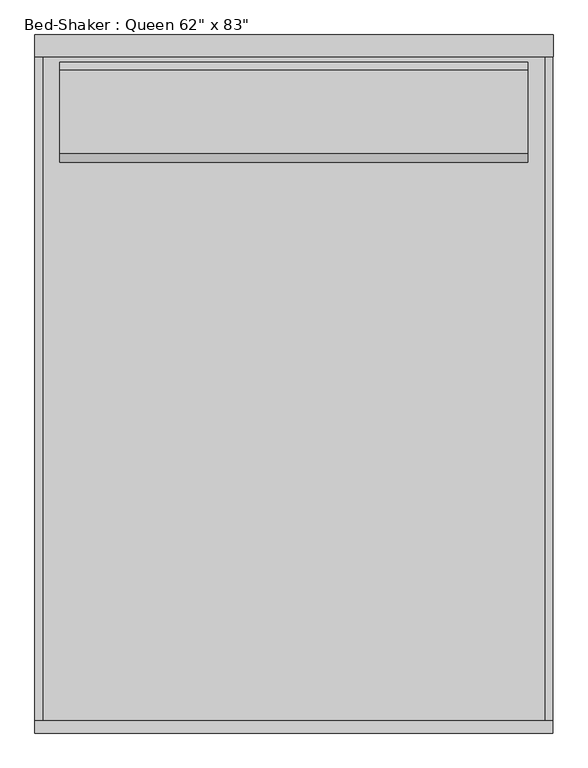
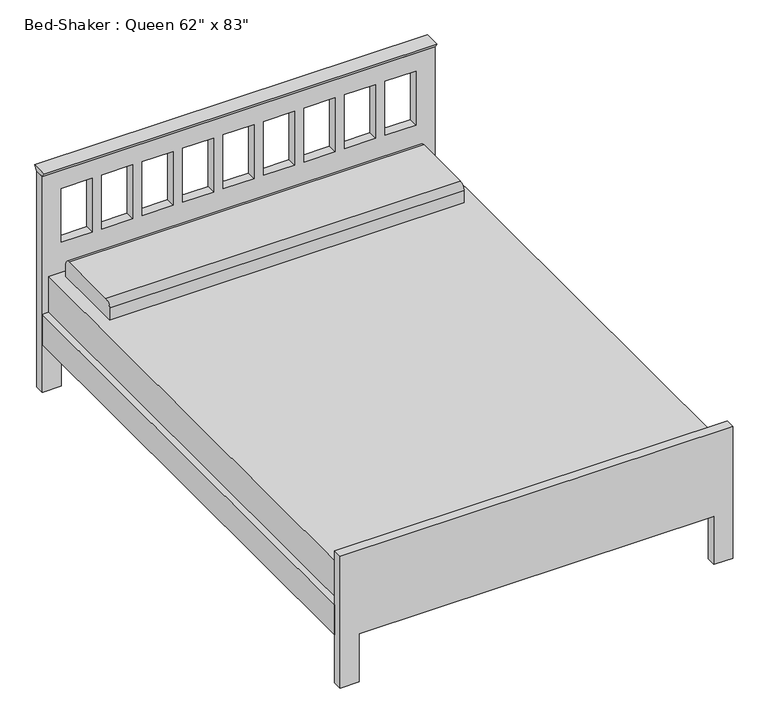
"""IFC4 building model written with IfcOpenShell, lengths in millimetres: furniture geometry."""

from ifc_helpers import new_model, si_unit, point, frame, frame_2d, origin, place, context, project, spatial, polyline, circle_curve, trimmed, segment, composite_curve, outline, extrude, source, transform, mapped, element, save


def furniture_35c09872(model_context):
    return source(origin(), model_context, "Body", "SweptSolid", [
        extrude(outline(polyline([(-38.1, 914.4), (-51.9545455, 933.45), (13.8545455, 933.45), (0.0, 914.4), (-38.1, 914.4)])), frame((-806.2365546, 0.0, 0.0), z_axis=(1.0, 0.0, 0.0), x_axis=(0.0, 1.0, 0.0)), (0.0, 0.0, 1.0), 1574.8533613),
        extrude(outline(composite_curve([segment(polyline([(-373.2486637, 482.6), (-373.2486637, 533.4)]), True, "CONTINUOUS"), segment(trimmed(circle_curve(frame_2d((-347.8486637, 533.4)), 25.4), [point((-373.2486637, 533.4))], [point((-347.8486637, 558.8))], False, "CARTESIAN"), True, "CONTINUOUS"), segment(polyline([(-347.8486637, 558.8), (-93.8486637, 558.8)]), True, "CONTINUOUS"), segment(trimmed(circle_curve(frame_2d((-93.8486637, 533.4)), 25.4), [point((-93.8486637, 558.8))], [point((-68.4486637, 533.4))], False, "CARTESIAN"), True, "CONTINUOUS"), segment(polyline([(-68.4486637, 533.4), (-68.4486637, 482.6), (-373.2486637, 482.6)]), True, "CONTINUOUS")], self_intersect=False)), frame((-730.25, 0.0, 0.0), z_axis=(1.0, 0.0, 0.0), x_axis=(0.0, 1.0, 0.0)), (0.0, 0.0, 1.0), 1422.4),
        extrude(outline(polyline([(742.95, -38.1), (742.95, -2070.1), (-781.05, -2070.1), (-781.05, -38.1), (742.95, -38.1)])), frame((0.0, 0.0, 228.6), z_axis=(0.0, 0.0, 1.0), x_axis=(1.0, 0.0, 0.0)), (0.0, 0.0, 1.0), 254.0),
        extrude(outline(polyline([(742.95, -2070.1), (742.95, -38.1), (768.35, -38.1), (768.35, -2070.1), (742.95, -2070.1)])), frame((0.0, 0.0, 203.0994861), z_axis=(0.0, 0.0, 1.0), x_axis=(1.0, 0.0, 0.0)), (0.0, 0.0, 1.0), 127.0),
        extrude(outline(polyline([(-806.45, -2070.1), (-806.45, -38.1), (-781.05, -38.1), (-781.05, -2070.1), (-806.45, -2070.1)])), frame((0.0, 0.0, 203.5755296), z_axis=(0.0, 0.0, 1.0), x_axis=(1.0, 0.0, 0.0)), (0.0, 0.0, 1.0), 127.0),
        extrude(outline(polyline([(0.0, -730.25), (203.2, -730.25), (203.2, 692.15), (0.0, 692.15), (0.0, 768.35), (558.8, 768.35), (558.8, -806.45), (0.0, -806.45), (0.0, -730.25)])), frame((0.0, -2108.2, 0.0), z_axis=(0.0, 1.0, 0.0), x_axis=(0.0, 0.0, 1.0)), (0.0, 0.0, 1.0), 38.1),
        extrude(outline(polyline([(914.4, 768.6168067), (914.4, -806.2365546), (0.0, -806.2365546), (0.0, -730.25), (203.2, -730.25), (203.2, 692.15), (0.0, 692.15), (0.0, 768.6168067), (914.4, 768.6168067)]), holes=[polyline([(838.2, -606.0722222), (609.6, -606.0722222), (609.6, -730.25), (838.2, -730.25), (838.2, -606.0722222)]), polyline([(838.2, -443.7944444), (609.6, -443.7944444), (609.6, -567.9722222), (838.2, -567.9722222), (838.2, -443.7944444)]), polyline([(838.2, -281.5166667), (609.6, -281.5166667), (609.6, -405.6944444), (838.2, -405.6944444), (838.2, -281.5166667)]), polyline([(838.2, -119.2388889), (609.6, -119.2388889), (609.6, -243.4166667), (838.2, -243.4166667), (838.2, -119.2388889)]), polyline([(838.2, 205.3166667), (609.6, 205.3166667), (609.6, 81.1388889), (838.2, 81.1388889), (838.2, 205.3166667)]), polyline([(838.2, 367.5944444), (609.6, 367.5944444), (609.6, 243.4166667), (838.2, 243.4166667), (838.2, 367.5944444)]), polyline([(838.2, 529.8722222), (609.6, 529.8722222), (609.6, 405.6944444), (838.2, 405.6944444), (838.2, 529.8722222)]), polyline([(838.2, 692.15), (609.6, 692.15), (609.6, 567.9722222), (838.2, 567.9722222), (838.2, 692.15)]), polyline([(838.2, 43.0388889), (609.6, 43.0388889), (609.6, -81.1388889), (838.2, -81.1388889), (838.2, 43.0388889)])]), frame((0.0, -38.1, 0.0), z_axis=(0.0, 1.0, 0.0), x_axis=(0.0, 0.0, 1.0)), (0.0, 0.0, 1.0), 38.1),
    ])


if __name__ == "__main__":
    model = new_model("IFC4")
    model_context = context("Model", 3, world=origin())
    ifc_project = project(units=[si_unit("LENGTHUNIT", "METRE", prefix="MILLI")], contexts=[model_context])
    site = spatial("IfcSite", under=ifc_project)
    building = spatial("IfcBuilding", under=site)
    placement = place(None, origin())
    furniture_shape = furniture_35c09872(model_context)
    element("IfcFurniture", 1, ObjectType="Bed-Shaker : Queen 62\" x 83\"", at=placement, inside=building, context=model_context, shape_type="MappedRepresentation", body=[
        mapped(furniture_shape, transform((0.0, 0.0, 0.0), x_axis=(1.0, 0.0, 0.0), y_axis=(0.0, 1.0, 0.0), z_axis=(0.0, 0.0, 1.0))),
    ])
    save(model, "model.ifc")

# Revit data of these elements
# Type "Bed-Shaker : Queen 62\" x 83\""
#   Assembly Code = "E2020200"
#   Length = 6' - 11"
#   Width = 5' - 2"
#   Frame Material = Birch
#   Mattress Material = Softwood, Lumber
#   Default Elevation = 0
# Element 1 (IfcFurniture, "Bed-Shaker : Queen 62\" x 83\"")
#   Materials on its faces: "Birch", "Softwood, Lumber"
# Materials
#   "Birch": class "Wood", colour RGB 210 159 95, transparency 0, Description = "Betula Alleghaniensis", Cost = 0
#   "Softwood, Lumber": class "Wood", colour RGB 223 192 134, transparency 0, Description = "Pinus Echinata", Cost = 0
